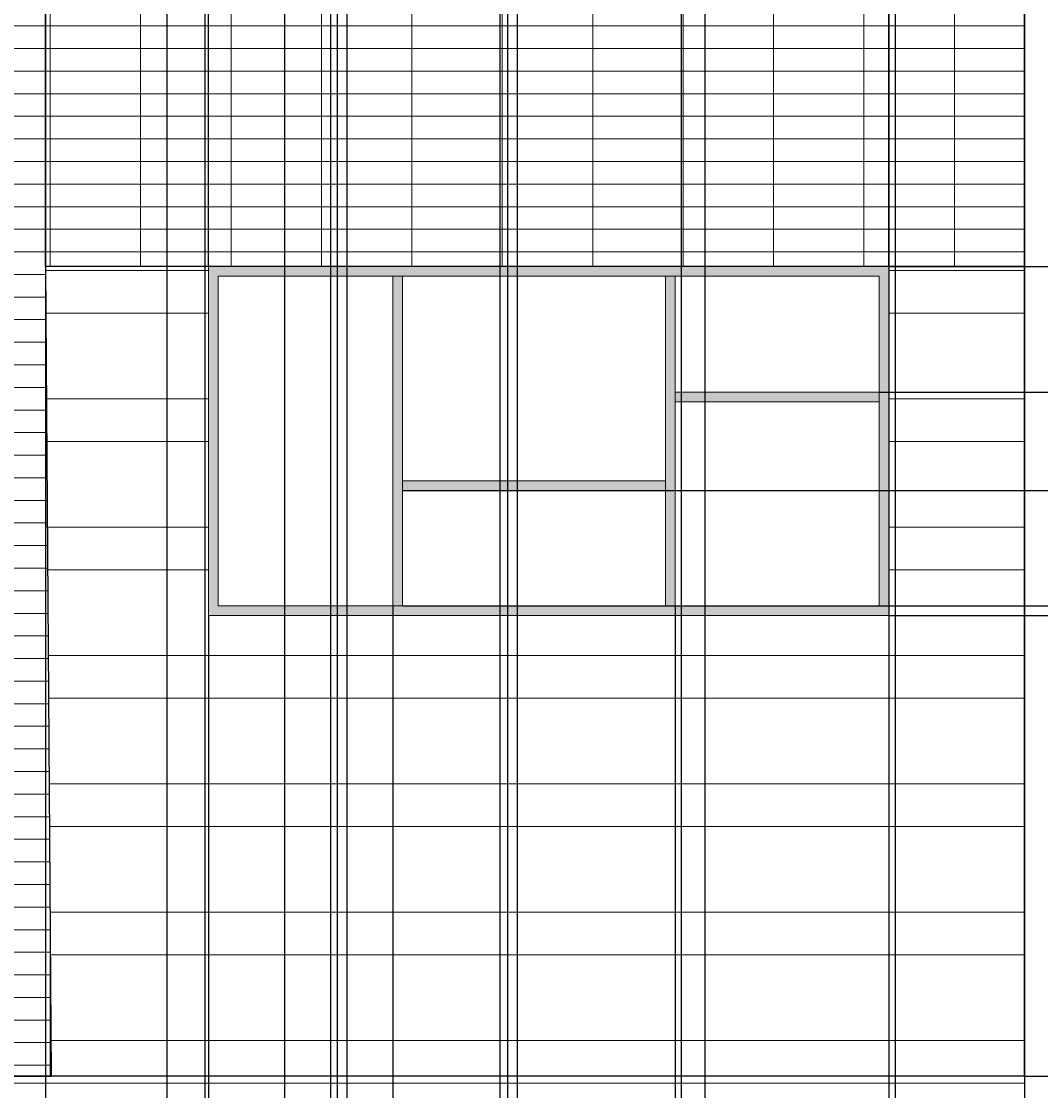
# Model space of a CAD drawing. Units: inches. Extents: x 241 to 943, y 109 to 1396.
# Tile 13 of 34: x 613 to 824, y 398 to 620. Entities that reach past the tile are written whole.
import ezdxf

# ---------------------------------------------------------------- set-up
doc = ezdxf.new("R2010")
doc.units = ezdxf.units.IN
doc.header["$MEASUREMENT"] = 0
for name, color, linetype, lineweight in [('A-ANNO-DIMS', 2, 'Continuous', 18), ('A-ELEV', 7, 'Continuous', 25), ('A-ELEV-SHAD', 9, 'Continuous', 13), ('A-GLAZ', 4, 'Continuous', 18), ('A-GLAZ-PATT', 18, 'Continuous', 13), ('A-WALL-PATT', 8, 'Continuous', 13)]:
    doc.layers.add(name, color=color, linetype=linetype, lineweight=lineweight)
doc.styles.get("Standard").update_dxf_attribs({"font": 'arial.ttf'})
doc.dimstyles.get("Standard").update_dxf_attribs({"dimtxt": 1.4375, "dimasz": 0.18, "dimexe": 0.18, "dimexo": 0.0625, "dimgap": 0.09, "dimtad": 0, "dimtih": 1, "dimtoh": 1, "dimdec": 4, "dimzin": 0, "dimdsep": 46, "dimlunit": 4, "dimtxsty": 'Standard', "dimcen": 0.09, "dimadec": 0, "dimazin": 0, "dimtfac": 1, "dimtdec": 4, "dimtofl": 0, "dimtmove": 0, "dimatfit": 3, "dimfxl": 1, "dimtolj": 1, "dimtzin": 0, "dimarcsym": 0})

# ---------------------------------------------------------------- blocks, each defined once
blk = doc.blocks.new('*D6')
at = {"layer": 'A-ANNO-DIMS', "color": 0, "lineweight": -2, "transparency": 16777216}
for p, q in [((820.84, 232.89), (820.84, 1395.05)), ((821.02, 1394.87), (848.73, 1394.87)), ((881.49, 1394.87), (853.77, 1394.87)), ((881.67, 232.89), (881.67, 1395.05))]:
    blk.add_line(p, q, dxfattribs=at)
at = {"layer": 'A-ANNO-DIMS', "color": 0, "transparency": 16777216}
for points in [[(821.02, 1394.9), (821.02, 1394.84), (820.84, 1394.87)], [(881.49, 1394.9), (881.49, 1394.84), (881.67, 1394.87)]]:
    blk.add_solid(points, dxfattribs=at)
at = {"layer": 'Defpoints', "color": 0, "transparency": 16777216}
for p in [(881.67, 1394.87), (820.84, 232.83), (881.67, 232.83)]:
    blk.add_point(p, dxfattribs=at)
at = {"layer": 'A-ANNO-DIMS', "color": 0, "transparency": 16777216, "insert": (851.25, 1394.87), "char_height": 1.438, "attachment_point": 5}
blk.add_mtext('\\A1;60.83', dxfattribs=at)
blk = doc.blocks.new('*D12')
at = {"layer": 'A-ANNO-DIMS', "color": 0, "lineweight": -2, "transparency": 16777216}
for p, q in [((530.23, 384.24), (530.23, 1395.05)), ((530.41, 1394.87), (587.56, 1394.87)), ((650.73, 1394.87), (593.58, 1394.87)), ((650.91, 384.24), (650.91, 1395.05))]:
    blk.add_line(p, q, dxfattribs=at)
at = {"layer": 'A-ANNO-DIMS', "color": 0, "transparency": 16777216}
for points in [[(530.41, 1394.9), (530.41, 1394.84), (530.23, 1394.87)], [(650.73, 1394.9), (650.73, 1394.84), (650.91, 1394.87)]]:
    blk.add_solid(points, dxfattribs=at)
at = {"layer": 'Defpoints', "color": 0, "transparency": 16777216}
for p in [(650.91, 1394.87), (530.23, 384.18), (650.91, 384.18)]:
    blk.add_point(p, dxfattribs=at)
at = {"layer": 'A-ANNO-DIMS', "color": 0, "transparency": 16777216, "insert": (590.57, 1394.87), "char_height": 1.438, "attachment_point": 5}
blk.add_mtext('\\A1;120.68', dxfattribs=at)
blk = doc.blocks.new('*D13')
at = {"layer": 'A-ANNO-DIMS', "color": 0, "lineweight": -2, "transparency": 16777216}
for p, q in [((650.91, 384.24), (650.91, 1395.05)), ((651.09, 1394.87), (656.14, 1394.87)), ((667.21, 1394.87), (662.16, 1394.87)), ((667.39, 290.06), (667.39, 1395.05))]:
    blk.add_line(p, q, dxfattribs=at)
at = {"layer": 'A-ANNO-DIMS', "color": 0, "transparency": 16777216}
for points in [[(651.09, 1394.9), (651.09, 1394.84), (650.91, 1394.87)], [(667.21, 1394.9), (667.21, 1394.84), (667.39, 1394.87)]]:
    blk.add_solid(points, dxfattribs=at)
at = {"layer": 'Defpoints', "color": 0, "transparency": 16777216}
for p in [(667.39, 1394.87), (650.91, 384.18), (667.39, 290)]:
    blk.add_point(p, dxfattribs=at)
at = {"layer": 'A-ANNO-DIMS', "color": 0, "transparency": 16777216, "insert": (659.15, 1394.87), "char_height": 1.438, "attachment_point": 5}
blk.add_mtext('\\A1;16.486', dxfattribs=at)
blk = doc.blocks.new('*D14')
at = {"layer": 'A-ANNO-DIMS', "color": 0, "lineweight": -2, "transparency": 16777216}
for p, q in [((667.39, 290.06), (667.39, 1395.05)), ((667.57, 1394.87), (727.7, 1394.87)), ((793.85, 1394.87), (733.72, 1394.87)), ((794.03, 290.06), (794.03, 1395.05))]:
    blk.add_line(p, q, dxfattribs=at)
at = {"layer": 'A-ANNO-DIMS', "color": 0, "transparency": 16777216}
for points in [[(667.57, 1394.9), (667.57, 1394.84), (667.39, 1394.87)], [(793.85, 1394.9), (793.85, 1394.84), (794.03, 1394.87)]]:
    blk.add_solid(points, dxfattribs=at)
at = {"layer": 'Defpoints', "color": 0, "transparency": 16777216}
for p in [(794.03, 1394.87), (667.39, 290), (794.03, 290)]:
    blk.add_point(p, dxfattribs=at)
at = {"layer": 'A-ANNO-DIMS', "color": 0, "transparency": 16777216, "insert": (730.71, 1394.87), "char_height": 1.438, "attachment_point": 5}
blk.add_mtext('\\A1;126.63', dxfattribs=at)
blk = doc.blocks.new('*D15')
at = {"layer": 'A-ANNO-DIMS', "color": 0, "lineweight": -2, "transparency": 16777216}
for p, q in [((794.03, 290.06), (794.03, 1395.05)), ((794.21, 1394.87), (805.04, 1394.87)), ((820.66, 1394.87), (809.82, 1394.87)), ((820.84, 232.89), (820.84, 1395.05))]:
    blk.add_line(p, q, dxfattribs=at)
at = {"layer": 'A-ANNO-DIMS', "color": 0, "transparency": 16777216}
for points in [[(794.21, 1394.9), (794.21, 1394.84), (794.03, 1394.87)], [(820.66, 1394.9), (820.66, 1394.84), (820.84, 1394.87)]]:
    blk.add_solid(points, dxfattribs=at)
at = {"layer": 'Defpoints', "color": 0, "transparency": 16777216}
for p in [(820.84, 1394.87), (794.03, 290), (820.84, 232.83)]:
    blk.add_point(p, dxfattribs=at)
at = {"layer": 'A-ANNO-DIMS', "color": 0, "transparency": 16777216, "insert": (807.43, 1394.87), "char_height": 1.438, "attachment_point": 5}
blk.add_mtext('\\A1;26.81', dxfattribs=at)
blk = doc.blocks.new('*D31')
at = {"layer": 'A-ANNO-DIMS', "color": 0, "lineweight": -2, "transparency": 16777216}
for p, q in [((792.75, 496.44), (940.6, 496.44)), ((940.42, 496.26), (940.42, 449.46)), ((940.42, 401.01), (940.42, 447.81)), ((820.9, 400.83), (940.6, 400.83))]:
    blk.add_line(p, q, dxfattribs=at)
at = {"layer": 'A-ANNO-DIMS', "color": 0, "transparency": 16777216}
for points in [[(940.39, 496.26), (940.45, 496.26), (940.42, 496.44)], [(940.39, 401.01), (940.45, 401.01), (940.42, 400.83)]]:
    blk.add_solid(points, dxfattribs=at)
at = {"layer": 'Defpoints', "color": 0, "transparency": 16777216}
for p in [(792.69, 496.44), (940.42, 496.44), (820.84, 400.83)]:
    blk.add_point(p, dxfattribs=at)
at = {"layer": 'A-ANNO-DIMS', "color": 0, "transparency": 16777216, "insert": (940.42, 448.63), "char_height": 1.438, "attachment_point": 5}
blk.add_mtext('\\A1;95.61', dxfattribs=at)
blk = doc.blocks.new('*D41')
at = {"layer": 'A-ANNO-DIMS', "color": 0, "lineweight": -2, "transparency": 16777216}
for p, q in [((820.77, 400.83), (244.31, 400.83)), ((244.49, 400.65), (244.49, 317.65)), ((244.49, 233.01), (244.49, 316.01)), ((820.77, 232.83), (244.31, 232.83))]:
    blk.add_line(p, q, dxfattribs=at)
at = {"layer": 'A-ANNO-DIMS', "color": 0, "transparency": 16777216}
for points in [[(244.46, 400.65), (244.52, 400.65), (244.49, 400.83)], [(244.46, 233.01), (244.52, 233.01), (244.49, 232.83)]]:
    blk.add_solid(points, dxfattribs=at)
at = {"layer": 'Defpoints', "color": 0, "transparency": 16777216}
for p in [(244.49, 400.83), (820.84, 400.83), (820.84, 232.83)]:
    blk.add_point(p, dxfattribs=at)
at = {"layer": 'A-ANNO-DIMS', "color": 0, "transparency": 16777216, "insert": (244.49, 316.83), "char_height": 1.438, "attachment_point": 5}
blk.add_mtext('\\A1;168', dxfattribs=at)
blk = doc.blocks.new('*D45')
at = {"layer": 'A-ANNO-DIMS', "color": 0, "lineweight": -2, "transparency": 16777216}
for p, q in [((792.75, 568.83), (940.6, 568.83)), ((940.42, 568.65), (940.42, 533.46)), ((940.42, 496.62), (940.42, 531.81)), ((792.75, 496.44), (940.6, 496.44))]:
    blk.add_line(p, q, dxfattribs=at)
at = {"layer": 'A-ANNO-DIMS', "color": 0, "transparency": 16777216}
for points in [[(940.39, 568.65), (940.45, 568.65), (940.42, 568.83)], [(940.39, 496.62), (940.45, 496.62), (940.42, 496.44)]]:
    blk.add_solid(points, dxfattribs=at)
at = {"layer": 'Defpoints', "color": 0, "transparency": 16777216}
for p in [(792.69, 568.83), (940.42, 568.83), (792.69, 496.44)]:
    blk.add_point(p, dxfattribs=at)
at = {"layer": 'A-ANNO-DIMS', "color": 0, "transparency": 16777216, "insert": (940.42, 532.63), "char_height": 1.438, "attachment_point": 5}
blk.add_mtext('\\A1;72.39', dxfattribs=at)
blk = doc.blocks.new('*D63')
at = {"layer": 'A-ANNO-DIMS', "color": 0, "lineweight": -2, "transparency": 16777216}
for p, q in [((651.6, 568.89), (651.6, 1395.05)), ((651.78, 1394.87), (719.84, 1394.87)), ((792.51, 1394.87), (724.45, 1394.87)), ((792.69, 568.89), (792.69, 1395.05))]:
    blk.add_line(p, q, dxfattribs=at)
at = {"layer": 'A-ANNO-DIMS', "color": 0, "transparency": 16777216}
for points in [[(651.78, 1394.9), (651.78, 1394.84), (651.6, 1394.87)], [(792.51, 1394.9), (792.51, 1394.84), (792.69, 1394.87)]]:
    blk.add_solid(points, dxfattribs=at)
at = {"layer": 'Defpoints', "color": 0, "transparency": 16777216}
for p in [(792.69, 1394.87), (651.6, 568.83), (792.69, 568.83)]:
    blk.add_point(p, dxfattribs=at)
at = {"layer": 'A-ANNO-DIMS', "color": 0, "transparency": 16777216, "insert": (722.14, 1394.87), "char_height": 1.438, "attachment_point": 5}
blk.add_mtext('\\A1;141.1', dxfattribs=at)
blk = doc.blocks.new('*D64')
at = {"layer": 'A-ANNO-DIMS', "color": 0, "lineweight": -2, "transparency": 16777216}
for p, q in [((792.69, 568.89), (792.69, 1395.05)), ((792.87, 1394.87), (803.68, 1394.87)), ((820.66, 1394.87), (809.85, 1394.87)), ((820.84, 568.89), (820.84, 1395.05))]:
    blk.add_line(p, q, dxfattribs=at)
at = {"layer": 'A-ANNO-DIMS', "color": 0, "transparency": 16777216}
for points in [[(792.87, 1394.9), (792.87, 1394.84), (792.69, 1394.87)], [(820.66, 1394.9), (820.66, 1394.84), (820.84, 1394.87)]]:
    blk.add_solid(points, dxfattribs=at)
at = {"layer": 'Defpoints', "color": 0, "transparency": 16777216}
for p in [(820.84, 1394.87), (792.69, 568.83), (820.84, 568.83)]:
    blk.add_point(p, dxfattribs=at)
at = {"layer": 'A-ANNO-DIMS', "color": 0, "transparency": 16777216, "insert": (806.76, 1394.87), "char_height": 1.438, "attachment_point": 5}
blk.add_mtext('\\A1;28.146', dxfattribs=at)
blk = doc.blocks.new('*D82')
at = {"layer": 'A-ANNO-DIMS', "color": 0, "lineweight": -2, "transparency": 16777216}
for p, q in [((565.2, 568.89), (565.2, 1395.05)), ((565.38, 1394.87), (605.89, 1394.87)), ((651.42, 1394.87), (610.91, 1394.87)), ((651.6, 568.89), (651.6, 1395.05))]:
    blk.add_line(p, q, dxfattribs=at)
at = {"layer": 'A-ANNO-DIMS', "color": 0, "transparency": 16777216}
for points in [[(565.38, 1394.9), (565.38, 1394.84), (565.2, 1394.87)], [(651.42, 1394.9), (651.42, 1394.84), (651.6, 1394.87)]]:
    blk.add_solid(points, dxfattribs=at)
at = {"layer": 'Defpoints', "color": 0, "transparency": 16777216}
for p in [(651.6, 1394.87), (565.2, 568.83), (651.6, 568.83)]:
    blk.add_point(p, dxfattribs=at)
at = {"layer": 'A-ANNO-DIMS', "color": 0, "transparency": 16777216, "insert": (608.4, 1394.87), "char_height": 1.438, "attachment_point": 5}
blk.add_mtext('\\A1;86.40', dxfattribs=at)
blk = doc.blocks.new('*D85')
at = {"layer": 'A-ANNO-DIMS', "color": 0, "lineweight": -2, "transparency": 16777216}
for p, q in [((749.7, 626.4), (940.6, 626.4)), ((940.42, 626.22), (940.42, 598.44)), ((940.42, 569.01), (940.42, 596.79)), ((792.75, 568.83), (940.6, 568.83))]:
    blk.add_line(p, q, dxfattribs=at)
at = {"layer": 'A-ANNO-DIMS', "color": 0, "transparency": 16777216}
for points in [[(940.39, 626.22), (940.45, 626.22), (940.42, 626.4)], [(940.39, 569.01), (940.45, 569.01), (940.42, 568.83)]]:
    blk.add_solid(points, dxfattribs=at)
at = {"layer": 'Defpoints', "color": 0, "transparency": 16777216}
for p in [(749.63, 626.4), (940.42, 626.4), (792.69, 568.83)]:
    blk.add_point(p, dxfattribs=at)
at = {"layer": 'A-ANNO-DIMS', "color": 0, "transparency": 16777216, "insert": (940.42, 597.62), "char_height": 1.438, "attachment_point": 5}
blk.add_mtext('\\A1;57.57', dxfattribs=at)
blk = doc.blocks.new('*D99')
at = {"layer": 'A-ANNO-DIMS', "color": 0, "lineweight": -2, "transparency": 16777216}
for p, q in [((417.09, 181.71), (417.09, 1395.05)), ((417.27, 1394.87), (539.16, 1394.87)), ((667.21, 1394.87), (545.33, 1394.87)), ((667.39, 214.58), (667.39, 1395.05))]:
    blk.add_line(p, q, dxfattribs=at)
at = {"layer": 'A-ANNO-DIMS', "color": 0, "transparency": 16777216}
for points in [[(417.27, 1394.9), (417.27, 1394.84), (417.09, 1394.87)], [(667.21, 1394.9), (667.21, 1394.84), (667.39, 1394.87)]]:
    blk.add_solid(points, dxfattribs=at)
at = {"layer": 'Defpoints', "color": 0, "transparency": 16777216}
for p in [(667.39, 1394.87), (667.39, 214.52), (417.09, 181.65)]:
    blk.add_point(p, dxfattribs=at)
at = {"layer": 'A-ANNO-DIMS', "color": 0, "transparency": 16777216, "insert": (542.24, 1394.87), "char_height": 1.438, "attachment_point": 5}
blk.add_mtext('\\A1;250.30', dxfattribs=at)
blk = doc.blocks.new('*D119')
at = {"layer": 'A-ANNO-DIMS', "color": 0, "lineweight": -2, "transparency": 16777216}
for p, q in [((617.76, 734.79), (617.76, 109.81)), ((642.92, 734.79), (642.92, 109.81)), ((617.94, 109.99), (627.81, 109.99)), ((642.74, 109.99), (632.87, 109.99))]:
    blk.add_line(p, q, dxfattribs=at)
at = {"layer": 'A-ANNO-DIMS', "color": 0, "transparency": 16777216}
for points in [[(617.94, 110.02), (617.94, 109.96), (617.76, 109.99)], [(642.74, 110.02), (642.74, 109.96), (642.92, 109.99)]]:
    blk.add_solid(points, dxfattribs=at)
at = {"layer": 'Defpoints', "color": 0, "transparency": 16777216}
for p in [(617.76, 734.85), (642.92, 734.85), (642.92, 109.99)]:
    blk.add_point(p, dxfattribs=at)
at = {"layer": 'A-ANNO-DIMS', "color": 0, "transparency": 16777216, "insert": (630.34, 109.99), "char_height": 1.438, "attachment_point": 5}
blk.add_mtext('\\A1;25.16', dxfattribs=at)
blk = doc.blocks.new('*D120')
at = {"layer": 'A-ANNO-DIMS', "color": 0, "lineweight": -2, "transparency": 16777216}
for p, q in [((642.92, 734.79), (642.92, 109.81)), ((678.27, 734.79), (678.27, 109.81)), ((643.1, 109.99), (658.07, 109.99)), ((678.09, 109.99), (663.11, 109.99))]:
    blk.add_line(p, q, dxfattribs=at)
at = {"layer": 'A-ANNO-DIMS', "color": 0, "transparency": 16777216}
for points in [[(643.1, 110.02), (643.1, 109.96), (642.92, 109.99)], [(678.09, 110.02), (678.09, 109.96), (678.27, 109.99)]]:
    blk.add_solid(points, dxfattribs=at)
at = {"layer": 'Defpoints', "color": 0, "transparency": 16777216}
for p in [(642.92, 734.85), (678.27, 734.85), (678.27, 109.99)]:
    blk.add_point(p, dxfattribs=at)
at = {"layer": 'A-ANNO-DIMS', "color": 0, "transparency": 16777216, "insert": (660.59, 109.99), "char_height": 1.438, "attachment_point": 5}
blk.add_mtext('\\A1;35.35', dxfattribs=at)
blk = doc.blocks.new('*D121')
at = {"layer": 'A-ANNO-DIMS', "color": 0, "lineweight": -2, "transparency": 16777216}
for p, q in [((680.27, 736.86), (680.27, 109.81)), ((713.62, 736.86), (713.62, 109.81)), ((680.45, 109.99), (693.87, 109.99)), ((713.44, 109.99), (700.02, 109.99))]:
    blk.add_line(p, q, dxfattribs=at)
at = {"layer": 'A-ANNO-DIMS', "color": 0, "transparency": 16777216}
for points in [[(680.45, 110.02), (680.45, 109.96), (680.27, 109.99)], [(713.44, 110.02), (713.44, 109.96), (713.62, 109.99)]]:
    blk.add_solid(points, dxfattribs=at)
at = {"layer": 'Defpoints', "color": 0, "transparency": 16777216}
for p in [(680.27, 736.92), (713.62, 736.92), (713.62, 109.99)]:
    blk.add_point(p, dxfattribs=at)
at = {"layer": 'A-ANNO-DIMS', "color": 0, "transparency": 16777216, "insert": (696.95, 109.99), "char_height": 1.438, "attachment_point": 5}
blk.add_mtext('\\A1;33.356', dxfattribs=at)
blk = doc.blocks.new('*D122')
at = {"layer": 'A-ANNO-DIMS', "color": 0, "lineweight": -2, "transparency": 16777216}
for p, q in [((715.62, 734.79), (715.62, 109.81)), ((754.54, 734.79), (754.54, 109.81)), ((715.8, 109.99), (732.7, 109.99)), ((754.36, 109.99), (737.46, 109.99))]:
    blk.add_line(p, q, dxfattribs=at)
at = {"layer": 'A-ANNO-DIMS', "color": 0, "transparency": 16777216}
for points in [[(715.8, 110.02), (715.8, 109.96), (715.62, 109.99)], [(754.36, 110.02), (754.36, 109.96), (754.54, 109.99)]]:
    blk.add_solid(points, dxfattribs=at)
at = {"layer": 'Defpoints', "color": 0, "transparency": 16777216}
for p in [(715.62, 734.85), (754.54, 734.85), (754.54, 109.99)]:
    blk.add_point(p, dxfattribs=at)
at = {"layer": 'A-ANNO-DIMS', "color": 0, "transparency": 16777216, "insert": (735.08, 109.99), "char_height": 1.438, "attachment_point": 5}
blk.add_mtext('\\A1;38.91', dxfattribs=at)
blk = doc.blocks.new('*D123')
at = {"layer": 'A-ANNO-DIMS', "color": 0, "lineweight": -2, "transparency": 16777216}
for p, q in [((754.54, 734.79), (754.54, 109.81)), ((792.69, 734.79), (792.69, 109.81)), ((754.72, 109.99), (771.09, 109.99)), ((792.51, 109.99), (776.13, 109.99))]:
    blk.add_line(p, q, dxfattribs=at)
at = {"layer": 'A-ANNO-DIMS', "color": 0, "transparency": 16777216}
for points in [[(754.72, 110.02), (754.72, 109.96), (754.54, 109.99)], [(792.51, 110.02), (792.51, 109.96), (792.69, 109.99)]]:
    blk.add_solid(points, dxfattribs=at)
at = {"layer": 'Defpoints', "color": 0, "transparency": 16777216}
for p in [(754.54, 734.85), (792.69, 734.85), (792.69, 109.99)]:
    blk.add_point(p, dxfattribs=at)
at = {"layer": 'A-ANNO-DIMS', "color": 0, "transparency": 16777216, "insert": (773.61, 109.99), "char_height": 1.438, "attachment_point": 5}
blk.add_mtext('\\A1;38.15', dxfattribs=at)
blk = doc.blocks.new('*D132')
at = {"layer": 'A-ANNO-DIMS', "color": 0, "lineweight": -2, "transparency": 16777216}
for p, q in [((676.87, 628.34), (676.87, 109.81)), ((617.76, 626.34), (617.76, 109.81)), ((617.94, 109.99), (644.94, 109.99)), ((676.69, 109.99), (649.69, 109.99))]:
    blk.add_line(p, q, dxfattribs=at)
at = {"layer": 'A-ANNO-DIMS', "color": 0, "transparency": 16777216}
for points in [[(617.94, 110.02), (617.94, 109.96), (617.76, 109.99)], [(676.69, 110.02), (676.69, 109.96), (676.87, 109.99)]]:
    blk.add_solid(points, dxfattribs=at)
at = {"layer": 'Defpoints', "color": 0, "transparency": 16777216}
for p in [(676.87, 628.4), (617.76, 626.4), (676.87, 109.99)]:
    blk.add_point(p, dxfattribs=at)
at = {"layer": 'A-ANNO-DIMS', "color": 0, "transparency": 16777216, "insert": (647.31, 109.99), "char_height": 1.438, "attachment_point": 5}
blk.add_mtext('\\A1;59.11', dxfattribs=at)
blk = doc.blocks.new('*D133')
at = {"layer": 'A-ANNO-DIMS', "color": 0, "lineweight": -2, "transparency": 16777216}
for p, q in [((676.87, 628.34), (676.87, 109.81)), ((712.02, 628.34), (712.02, 109.81)), ((677.05, 109.99), (691.92, 109.99)), ((711.84, 109.99), (696.96, 109.99))]:
    blk.add_line(p, q, dxfattribs=at)
at = {"layer": 'A-ANNO-DIMS', "color": 0, "transparency": 16777216}
for points in [[(677.05, 110.02), (677.05, 109.96), (676.87, 109.99)], [(711.84, 110.02), (711.84, 109.96), (712.02, 109.99)]]:
    blk.add_solid(points, dxfattribs=at)
at = {"layer": 'Defpoints', "color": 0, "transparency": 16777216}
for p in [(676.87, 628.4), (712.02, 628.4), (712.02, 109.99)]:
    blk.add_point(p, dxfattribs=at)
at = {"layer": 'A-ANNO-DIMS', "color": 0, "transparency": 16777216, "insert": (694.44, 109.99), "char_height": 1.438, "attachment_point": 5}
blk.add_mtext('\\A1;35.15', dxfattribs=at)
blk = doc.blocks.new('*D134')
at = {"layer": 'A-ANNO-DIMS', "color": 0, "lineweight": -2, "transparency": 16777216}
for p, q in [((712.02, 628.34), (712.02, 109.81)), ((749.63, 626.34), (749.63, 109.81)), ((712.2, 109.99), (727.75, 109.99)), ((749.45, 109.99), (733.9, 109.99))]:
    blk.add_line(p, q, dxfattribs=at)
at = {"layer": 'A-ANNO-DIMS', "color": 0, "transparency": 16777216}
for points in [[(712.2, 110.02), (712.2, 109.96), (712.02, 109.99)], [(749.45, 110.02), (749.45, 109.96), (749.63, 109.99)]]:
    blk.add_solid(points, dxfattribs=at)
at = {"layer": 'Defpoints', "color": 0, "transparency": 16777216}
for p in [(712.02, 628.4), (749.63, 626.4), (749.63, 109.99)]:
    blk.add_point(p, dxfattribs=at)
at = {"layer": 'A-ANNO-DIMS', "color": 0, "transparency": 16777216, "insert": (730.82, 109.99), "char_height": 1.438, "attachment_point": 5}
blk.add_mtext('\\A1;37.616', dxfattribs=at)
blk = doc.blocks.new('*D142')
at = {"layer": 'A-ANNO-DIMS', "color": 0, "lineweight": -2, "transparency": 16777216}
for p, q in [((689.79, 498.38), (689.79, 109.81)), ((651.6, 496.38), (651.6, 109.81)), ((651.78, 109.99), (668.18, 109.99)), ((689.61, 109.99), (673.21, 109.99))]:
    blk.add_line(p, q, dxfattribs=at)
at = {"layer": 'A-ANNO-DIMS', "color": 0, "transparency": 16777216}
for points in [[(651.78, 110.02), (651.78, 109.96), (651.6, 109.99)], [(689.61, 110.02), (689.61, 109.96), (689.79, 109.99)]]:
    blk.add_solid(points, dxfattribs=at)
at = {"layer": 'Defpoints', "color": 0, "transparency": 16777216}
for p in [(689.79, 498.44), (651.6, 496.44), (689.79, 109.99)]:
    blk.add_point(p, dxfattribs=at)
at = {"layer": 'A-ANNO-DIMS', "color": 0, "transparency": 16777216, "insert": (670.7, 109.99), "char_height": 1.438, "attachment_point": 5}
blk.add_mtext('\\A1;38.20', dxfattribs=at)
blk = doc.blocks.new('*D143')
at = {"layer": 'A-ANNO-DIMS', "color": 0, "lineweight": -2, "transparency": 16777216}
for p, q in [((689.79, 498.38), (689.79, 109.81)), ((748.33, 498.38), (748.33, 109.81)), ((689.97, 109.99), (716.55, 109.99)), ((748.15, 109.99), (721.58, 109.99))]:
    blk.add_line(p, q, dxfattribs=at)
at = {"layer": 'A-ANNO-DIMS', "color": 0, "transparency": 16777216}
for points in [[(689.97, 110.02), (689.97, 109.96), (689.79, 109.99)], [(748.15, 110.02), (748.15, 109.96), (748.33, 109.99)]]:
    blk.add_solid(points, dxfattribs=at)
at = {"layer": 'Defpoints', "color": 0, "transparency": 16777216}
for p in [(689.79, 498.44), (748.33, 498.44), (748.33, 109.99)]:
    blk.add_point(p, dxfattribs=at)
at = {"layer": 'A-ANNO-DIMS', "color": 0, "transparency": 16777216, "insert": (719.06, 109.99), "char_height": 1.438, "attachment_point": 5}
blk.add_mtext('\\A1;58.54', dxfattribs=at)
blk = doc.blocks.new('*D144')
at = {"layer": 'A-ANNO-DIMS', "color": 0, "lineweight": -2, "transparency": 16777216}
for p, q in [((748.33, 498.38), (748.33, 109.81)), ((792.69, 496.38), (792.69, 109.81)), ((748.51, 109.99), (767.97, 109.99)), ((792.51, 109.99), (773.06, 109.99))]:
    blk.add_line(p, q, dxfattribs=at)
at = {"layer": 'A-ANNO-DIMS', "color": 0, "transparency": 16777216}
for points in [[(748.51, 110.02), (748.51, 109.96), (748.33, 109.99)], [(792.51, 110.02), (792.51, 109.96), (792.69, 109.99)]]:
    blk.add_solid(points, dxfattribs=at)
at = {"layer": 'Defpoints', "color": 0, "transparency": 16777216}
for p in [(748.33, 498.44), (792.69, 496.44), (792.69, 109.99)]:
    blk.add_point(p, dxfattribs=at)
at = {"layer": 'A-ANNO-DIMS', "color": 0, "transparency": 16777216, "insert": (770.51, 109.99), "char_height": 1.438, "attachment_point": 5}
blk.add_mtext('\\A1;44.36', dxfattribs=at)
blk = doc.blocks.new('*D145')
at = {"layer": 'A-ANNO-DIMS', "color": 0, "lineweight": -2, "transparency": 16777216}
for p, q in [((691.86, 522.37), (940.6, 522.37)), ((940.42, 522.19), (940.42, 511.23)), ((940.42, 498.62), (940.42, 509.58)), ((691.86, 498.44), (940.6, 498.44))]:
    blk.add_line(p, q, dxfattribs=at)
at = {"layer": 'A-ANNO-DIMS', "color": 0, "transparency": 16777216}
for points in [[(940.39, 522.19), (940.45, 522.19), (940.42, 522.37)], [(940.39, 498.62), (940.45, 498.62), (940.42, 498.44)]]:
    blk.add_solid(points, dxfattribs=at)
at = {"layer": 'Defpoints', "color": 0, "transparency": 16777216}
for p in [(691.79, 522.37), (940.42, 522.37), (691.79, 498.44)]:
    blk.add_point(p, dxfattribs=at)
at = {"layer": 'A-ANNO-DIMS', "color": 0, "transparency": 16777216, "insert": (940.42, 510.41), "char_height": 1.438, "attachment_point": 5}
blk.add_mtext('\\A1;23.933', dxfattribs=at)
blk = doc.blocks.new('*D146')
at = {"layer": 'A-ANNO-DIMS', "color": 0, "lineweight": -2, "transparency": 16777216}
for p, q in [((790.75, 542.8), (940.6, 542.8)), ((940.42, 542.62), (940.42, 521.44)), ((940.42, 498.62), (940.42, 519.8)), ((790.75, 498.44), (940.6, 498.44))]:
    blk.add_line(p, q, dxfattribs=at)
at = {"layer": 'A-ANNO-DIMS', "color": 0, "transparency": 16777216}
for points in [[(940.39, 542.62), (940.45, 542.62), (940.42, 542.8)], [(940.39, 498.62), (940.45, 498.62), (940.42, 498.44)]]:
    blk.add_solid(points, dxfattribs=at)
at = {"layer": 'Defpoints', "color": 0, "transparency": 16777216}
for p in [(790.69, 542.8), (940.42, 542.8), (790.69, 498.44)]:
    blk.add_point(p, dxfattribs=at)
at = {"layer": 'A-ANNO-DIMS', "color": 0, "transparency": 16777216, "insert": (940.42, 520.62), "char_height": 1.438, "attachment_point": 5}
blk.add_mtext('\\A1;44.36', dxfattribs=at)

msp = doc.modelspace()

# ---------------------------------------------------------------- hatches: boundary and pattern name
at = {"layer": 'A-ELEV-SHAD'}
h = msp.add_hatch(color=256, dxfattribs=at)
h.dxf.hatch_style = 1
h.paths.add_polyline_path([(748.3325, 566.8295), (746.3325, 566.8295), (746.3325, 498.4395), (748.3325, 498.4395)])
h.paths.add_polyline_path([(746.3325, 524.3723), (691.794, 524.3723), (691.794, 522.3723), (746.3325, 522.3723)])
h.paths.add_polyline_path([(691.794, 566.8295), (689.794, 566.8295), (689.794, 498.4395), (691.794, 498.4395)])
h.paths.add_polyline_path([(790.691, 542.7994), (748.3325, 542.7994), (748.3325, 540.7994), (790.691, 540.7994)])
h.paths.add_polyline_path([(500.3323, 384.1784), (479.596, 384.1784), (479.596, 289.6933), (500.3323, 289.6933)])
h.paths.add_polyline_path([(481.596, 291.6933), (481.596, 382.1784), (498.3323, 382.1784), (498.3323, 291.6933)], flags=16)
h.paths.add_polyline_path([(462.1074, 384.1784), (390.895, 384.1784), (390.895, 289.6933), (462.1074, 289.6933)])
h.paths.add_polyline_path([(392.895, 291.6933), (392.895, 382.1784), (460.1074, 382.1784), (460.1074, 291.6933)], flags=16)
h.paths.add_polyline_path([(794.0275, 289.9984), (667.3935, 289.9984), (667.3935, 214.5189), (794.0275, 214.5189)])
h.paths.add_polyline_path([(792.0275, 287.9984), (792.0275, 216.5189), (669.3935, 216.5189), (669.3935, 287.9984)], flags=16)
h.paths.add_polyline_path([(508.0803, 525.3816), (506.0803, 525.3816), (506.0803, 521.3754), (452.9259, 521.3754), (452.9259, 525.3816), (450.9259, 525.3816), (450.9259, 519.3754), (508.0803, 519.3754)], flags=0)
h.paths.add_polyline_path([(508.0803, 566.8295), (450.9259, 566.8295), (450.9259, 527.3816), (452.9259, 527.3816), (452.9259, 564.8295), (506.0803, 564.8295), (506.0803, 527.3816), (508.0803, 527.3816)], flags=0)
h.paths.add_polyline_path([(537.4269, 566.8295), (534.1778, 566.8295), (534.1778, 527.3816), (537.4269, 527.3816)], flags=0)
h.paths.add_polyline_path([(537.4269, 525.3816), (534.1778, 525.3816), (534.1778, 508.9074), (537.4269, 508.9074)], flags=0)
h.paths.add_polyline_path([(565.2023, 568.8295), (424.1086, 568.8295), (424.1086, 496.4395), (565.2023, 496.4395)])
h.paths.add_polyline_path([(563.2023, 508.9074), (563.2023, 498.4395), (426.1086, 498.4395), (426.1086, 566.8295), (563.2023, 566.8295)], flags=16)
h.paths.add_polyline_path([(508.0803, 508.9074), (508.0803, 519.3754), (450.9259, 519.3754), (450.9259, 525.3816), (445.5808, 525.3816, -1), (445.5808, 527.3816), (450.9259, 527.3816), (450.9259, 566.8295), (508.0803, 566.8295), (537.4269, 566.8295), (537.4269, 508.9074)], flags=0)
h.paths.add_polyline_path([(506.0803, 521.3754), (452.9259, 521.3754), (452.9259, 564.8295), (506.0803, 564.8295)], flags=0)
h = msp.add_hatch(color=256, dxfattribs=at)
h.dxf.hatch_style = 1
h.paths.add_polyline_path([(691.794, 566.8295), (689.794, 566.8295), (689.794, 498.4395), (691.794, 498.4395)], flags=0)
h.paths.add_polyline_path([(792.691, 568.8295), (651.5974, 568.8295), (651.5974, 496.4395), (792.691, 496.4395)])
h.paths.add_polyline_path([(790.691, 566.8295), (790.691, 498.4395), (653.5974, 498.4395), (653.5974, 566.8295)], flags=16)
h.paths.add_polyline_path([(691.794, 524.3723), (746.3325, 524.3723), (746.3325, 522.3723), (691.794, 522.3723)], flags=0)
h.paths.add_polyline_path([(746.3325, 524.3723), (691.794, 524.3723), (691.794, 522.3723), (746.3325, 522.3723)], flags=0)
h.paths.add_polyline_path([(748.3325, 566.8295), (746.3325, 566.8295), (746.3325, 498.4395), (748.3325, 498.4395)], flags=0)
at = {"layer": 'A-GLAZ-PATT'}
h = msp.add_hatch(dxfattribs=at)
h.set_pattern_fill('ANSI31', color=256, scale=34, angle=45)
h.paths.add_polyline_path([(486.3418, 786.9154), (413.1187, 786.9154), (413.1187, 761.2284), (486.3418, 761.2284)])
h.paths.add_polyline_path([(486.3418, 954.9154), (413.1187, 954.9154), (413.1187, 929.2284), (486.3418, 929.2284)])
h.paths.add_polyline_path([(462.1074, 289.6933), (390.895, 289.6933), (390.895, 277.4626), (390.895, 274.3507), (462.1074, 274.3507), (462.1074, 277.4626)])
h.paths.add_polyline_path([(500.3323, 289.6933), (479.596, 289.6933), (479.596, 274.3507), (500.3323, 274.3507)])
h.paths.add_polyline_path([(450.9259, 566.8295), (426.1086, 566.8295), (426.1086, 498.4395), (446.4348, 498.4395), (446.4348, 519.3754), (450.9259, 519.3754), (450.9259, 525.3816), (445.5808, 525.3816, -1), (445.5808, 527.3816), (450.9259, 527.3816)])
h.paths.add_polyline_path([(563.2023, 508.9074), (534.1778, 508.9074), (508.1906, 508.9074), (508.1906, 498.4395), (563.2023, 498.4395)])
h.paths.add_polyline_path([(747.6328, 700.7912), (712.0171, 700.7912), (712.0171, 628.4013), (747.6328, 628.4013)])
h.paths.add_polyline_path([(446.4348, 643.7483), (426.1086, 643.7483), (426.1086, 630.4013), (446.4348, 630.4013)])
h.paths.add_polyline_path([(564.8076, 841.5382), (553.5166, 841.5382), (508.3064, 841.5382), (508.3064, 782.5808), (564.8076, 782.5808)])
h.paths.add_polyline_path([(564.8076, 780.5808), (508.3064, 780.5808), (508.3064, 773.4916), (564.8076, 773.4916)])
h.paths.add_polyline_path([(792.691, 762.5799), (759.6248, 762.5799), (759.6248, 736.9235), (759.6248, 734.8538), (792.691, 734.8538)])
h.paths.add_polyline_path([(564.8076, 1009.5382), (553.5166, 1009.5382), (508.3064, 1009.5382), (508.3064, 950.5808), (562.3033, 950.5808, -1), (562.3033, 948.5808), (508.3064, 948.5808), (508.3064, 941.4916), (564.8076, 941.4916)])
h.paths.add_polyline_path([(486.3418, 1122.9154), (413.1187, 1122.9154), (413.1187, 1097.2284), (486.3418, 1097.2284)])
at = {"layer": 'A-WALL-PATT'}
h = msp.add_hatch(dxfattribs=at)
h.set_pattern_fill('GRATE', color=256, scale=150)
h.paths.add_polyline_path([(747.7579, 1238.8538), (747.7579, 1275.9142), (747.7579, 1336.1154), (508.3064, 1336.1154), (508.3064, 1275.9142), (508.3064, 1238.8538), (508.3064, 1177.5382), (508.3064, 1109.4916), (508.3064, 1070.8538), (553.5166, 1070.8538), (749.6328, 1070.8538)])
h.paths.add_polyline_path([(533.952, 1108.1686), (533.952, 1177.7336), (533.952, 1303.0286), (724.819, 1303.0286), (724.819, 1108.1686)], flags=16)
h.paths.add_polyline_path([(535.952, 1110.1686), (535.952, 1175.7336), (722.819, 1175.7336), (722.819, 1110.1686)], flags=0)
h.paths.add_polyline_path([(643.4534, 1134.0739), (622.521, 1134.0739), (622.521, 1136.0739), (643.4534, 1136.0739)], flags=0)
h.paths.add_polyline_path([(617.7594, 568.8295), (617.7594, 734.8538), (377.0391, 734.8538), (377.0391, 566.8538), (377.0391, 400.8295), (417.0913, 400.8295), (618.9643, 400.8295)])
h.paths.add_polyline_path([(424.1086, 496.4395), (424.1086, 568.8295), (565.2023, 568.8295), (565.2023, 496.4395)], flags=16)
h.paths.add_polyline_path([(426.1086, 498.4395), (426.1086, 566.8295), (563.2023, 566.8295), (563.2023, 508.9074), (563.2023, 498.4395)], flags=0)
h.paths.add_polyline_path([(508.0803, 508.9074), (508.0803, 519.3754), (450.9259, 519.3754), (450.9259, 525.3816), (445.5808, 525.3816, -1), (445.5808, 527.3816), (450.9259, 527.3816), (450.9259, 566.8295), (508.0803, 566.8295), (537.4269, 566.8295), (537.4269, 508.9074)], flags=0)
h.paths.add_polyline_path([(506.0803, 521.3754), (452.9259, 521.3754), (452.9259, 564.8295), (506.0803, 564.8295)], flags=0)
h.paths.add_polyline_path([(424.1086, 628.4013), (424.1086, 700.7912), (592.9542, 700.7912), (592.9542, 628.4013)], flags=16)
h.paths.add_polyline_path([(426.1086, 630.4013), (426.1086, 698.7912), (590.8792, 698.7912), (590.8792, 630.4013)], flags=0)
h.paths.add_polyline_path([(508.1906, 651.3371), (508.0803, 651.3371), (450.9259, 651.3371), (428.0291, 651.3371), (428.0291, 698.7912), (451.9767, 698.7912), (508.0803, 698.7912), (537.4269, 698.7912), (563.2023, 698.7912), (563.2023, 659.3434), (563.9297, 659.3434), (563.9297, 651.3371)], flags=0)
h.paths.add_polyline_path([(506.0803, 653.3371), (452.9259, 653.3371), (452.9259, 657.3434), (445.5808, 657.3434, -1), (445.5808, 659.3434), (452.9259, 659.3434), (452.9259, 696.7912), (506.0803, 696.7912)], flags=0)
h = msp.add_hatch(dxfattribs=at)
h.set_pattern_fill('GRATE', color=256, scale=150)
h.paths.add_polyline_path([(820.8374, 1070.8538), (749.6328, 1070.8538), (553.5166, 1070.8538), (508.3064, 1070.8538), (508.3064, 1009.5382), (553.5166, 1009.5382), (564.8076, 1009.5382), (603.8694, 1009.5382), (751.5078, 1009.5382), (751.5078, 902.8538), (603.8694, 902.8538), (603.8694, 1009.5382), (564.8076, 1009.5382), (564.8076, 941.4916), (568.1348, 941.4916), (568.1348, 902.8538), (581.3632, 902.8538), (581.3632, 841.5382), (564.8076, 841.5382), (564.8076, 782.5808), (605.9087, 782.5808, -1), (605.9087, 780.5808), (564.8076, 780.5808), (564.8076, 773.4916), (597.514, 773.4916), (607.8162, 773.4916), (607.8162, 734.8538), (617.7594, 734.8538), (617.7594, 841.5382), (792.691, 841.5382), (792.691, 734.8538), (617.7594, 734.8538), (617.7594, 702.7912), (749.6328, 702.7912), (749.6328, 626.4013), (617.7594, 626.4013), (617.7594, 568.8295), (820.8374, 568.8295), (820.8374, 736.8295), (820.8374, 902.8538)])
h = msp.add_hatch(dxfattribs=at)
h.set_pattern_fill('ANSI32', color=256, scale=71, angle=135)
h.paths.add_polyline_path([(820.8374, 568.8295), (792.691, 568.8295), (792.691, 496.4395), (651.5974, 496.4395), (651.5974, 568.8295), (617.7594, 568.8295), (618.9643, 400.8295), (417.0913, 400.8295), (377.0391, 400.8295), (377.0391, 398.8538), (377.0391, 396.8782), (377.0391, 228.8782), (377.0391, 177.6977), (416.5078, 181.5724), (417.0913, 181.649), (530.2303, 196.5065), (530.2303, 384.1784), (650.907, 384.1784), (651.7861, 212.4693), (667.3935, 214.5189), (667.3935, 289.9984), (794.0275, 289.9984), (794.0275, 232.8295), (820.8374, 232.8295), (820.8374, 400.8295)])
h.paths.add_polyline_path([(500.3323, 384.1784), (500.3323, 289.6933), (500.3323, 274.3507), (479.596, 274.3507), (479.596, 289.6933), (479.596, 384.1784)], flags=16)
h.paths.add_polyline_path([(498.3323, 382.1784), (498.3323, 291.6933), (481.596, 291.6933), (481.596, 382.1784)], flags=0)
h.paths.add_polyline_path([(462.1074, 384.1784), (462.1074, 289.6933), (462.1074, 277.4626), (462.1074, 274.3507), (390.895, 274.3507), (390.895, 277.4626), (390.895, 289.6933), (390.895, 384.1784)], flags=16)
h.paths.add_polyline_path([(460.1074, 382.1784), (460.1074, 291.6933), (392.895, 291.6933), (392.895, 382.1784)], flags=0)
h.paths.add_polyline_path([(595.3136, 372.9401), (641.6196, 372.9401), (641.6196, 246.4081), (651.6121, 246.4593), (650.907, 384.1784), (530.2303, 384.1784), (530.2303, 245.8378), (595.3136, 246.1711)], flags=17)

# ---------------------------------------------------------------- linework, layer by layer
at = {"layer": 'A-ELEV'}
for p, q in [((820.8374, 568.8295), (820.8374, 736.8295)), ((617.7594, 568.8295), (617.7594, 734.8538)), ((820.8374, 568.8295), (617.7594, 568.8295)), ((617.7594, 568.8295), (618.9643, 400.8295)), ((820.8374, 400.8295), (820.8374, 568.8295)), ((417.0913, 400.8295), (618.9643, 400.8295)), ((820.8374, 400.8295), (820.8374, 232.8295))]:
    msp.add_line(p, q, dxfattribs=at)
at = {"layer": 'A-GLAZ'}
for p, q in [((689.794, 566.8295), (689.794, 498.4395)), ((691.794, 566.8295), (691.794, 498.4395)), ((746.3325, 566.8295), (746.3325, 498.4395)), ((748.3325, 566.8295), (748.3325, 498.4395)), ((748.3325, 542.7994), (790.691, 542.7994)), ((748.3325, 540.7994), (790.691, 540.7994)), ((691.794, 524.3723), (746.3325, 524.3723)), ((691.794, 522.3723), (746.3325, 522.3723))]:
    msp.add_line(p, q, dxfattribs=at)
for points in [[(651.5974, 568.8295), (792.691, 568.8295), (792.691, 496.4395), (651.5974, 496.4395)], [(653.5974, 566.8295), (790.691, 566.8295), (790.691, 498.4395), (653.5974, 498.4395)]]:
    msp.add_lwpolyline(points, close=True, dxfattribs=at)

# ---------------------------------------------------------------- dimensions: what is measured, and where the dimension line sits
at = {"layer": 'A-ANNO-DIMS'}
for base, p1, p2, override, picture, middle in [((667.3935, 1394.8654), (417.0913, 181.649), (667.3935, 214.5189), {"dimdec": 2, "dimlfac": 1, "dimrnd": 0, "dimzin": 0, "dimdsep": 46, "dimlunit": 2}, '*D99', (542.2424, 1394.8654)), ((650.907, 1394.8654), (530.2303, 384.1784), (650.907, 384.1784), {"dimdec": 2, "dimlfac": 1, "dimrnd": 0, "dimzin": 0, "dimdsep": 46, "dimlunit": 2}, '*D12', (590.5686, 1394.8654)), ((651.5974, 1394.8654), (565.2023, 568.8295), (651.5974, 568.8295), {"dimdec": 2, "dimlfac": 1, "dimrnd": 0, "dimzin": 0, "dimdsep": 46, "dimlunit": 2}, '*D82', (608.3998, 1394.8654)), ((667.39345, 1394.86544), (650.90697, 384.17836), (667.39345, 289.99842), {"dimdec": 3, "dimlfac": 1, "dimrnd": 0, "dimzin": 0, "dimdsep": 46, "dimlunit": 2}, '*D13', (659.15021, 1394.86544)), ((792.691, 1394.8654), (651.5974, 568.8295), (792.691, 568.8295), {"dimdec": 1, "dimlfac": 1, "dimrnd": 0, "dimzin": 0, "dimdsep": 46, "dimlunit": 2}, '*D63', (722.1442, 1394.8654)), ((794.0275, 1394.8654), (667.3935, 289.9984), (794.0275, 289.9984), {"dimdec": 2, "dimlfac": 1, "dimrnd": 0, "dimzin": 0, "dimdsep": 46, "dimlunit": 2}, '*D14', (730.7105, 1394.8654)), ((820.8374, 1394.8654), (792.691, 568.8295), (820.8374, 568.8295), {"dimdec": 3, "dimlfac": 1, "dimrnd": 0, "dimzin": 0, "dimdsep": 46, "dimlunit": 2}, '*D64', (806.7642, 1394.8654)), ((820.8374, 1394.8654), (794.0275, 289.9984), (820.8374, 232.8295), {"dimdec": 2, "dimlfac": 1, "dimrnd": 0, "dimzin": 0, "dimdsep": 46, "dimlunit": 2}, '*D15', (807.4324, 1394.8654)), ((881.667, 1394.8654), (820.8374, 232.8295), (881.667, 232.8295), {"dimdec": 2, "dimlfac": 1, "dimrnd": 0, "dimzin": 0, "dimdsep": 46, "dimlunit": 2}, '*D6', (851.2522, 1394.8654)), ((713.6236, 109.9907), (680.2674, 736.9235), (713.6236, 736.9235), {"dimdec": 3, "dimlfac": 1, "dimrnd": 0, "dimzin": 0, "dimdsep": 46, "dimlunit": 2}, '*D121', (696.9455, 109.9907)), ((642.9197, 109.9907), (617.7594, 734.8538), (642.9197, 734.8538), {"dimdec": 2, "dimlfac": 1, "dimrnd": 0, "dimzin": 0, "dimdsep": 46, "dimlunit": 2}, '*D119', (630.3395, 109.9907)), ((678.2674, 109.9907), (642.9197, 734.8538), (678.2674, 734.8538), {"dimdec": 2, "dimlfac": 1, "dimrnd": 0, "dimzin": 0, "dimdsep": 46, "dimlunit": 2}, '*D120', (660.5935, 109.9907)), ((754.5373, 109.9907), (715.6236, 734.8538), (754.5373, 734.8538), {"dimdec": 2, "dimlfac": 1, "dimrnd": 0, "dimzin": 0, "dimdsep": 46, "dimlunit": 2}, '*D122', (735.0804, 109.9907)), ((792.691, 109.9907), (754.5373, 734.8538), (792.691, 734.8538), {"dimdec": 2, "dimlfac": 1, "dimrnd": 0, "dimzin": 0, "dimdsep": 46, "dimlunit": 2}, '*D123', (773.6142, 109.9907)), ((676.8698, 109.9907), (617.7594, 626.4013), (676.8698, 628.4013), {"dimdec": 2, "dimlfac": 1, "dimrnd": 0, "dimzin": 0, "dimdsep": 46, "dimlunit": 2}, '*D132', (647.3146, 109.9907)), ((712.0171, 109.9907), (676.8698, 628.4013), (712.0171, 628.4013), {"dimdec": 2, "dimlfac": 1, "dimrnd": 0, "dimzin": 0, "dimdsep": 46, "dimlunit": 2}, '*D133', (694.4435, 109.9907)), ((749.6328, 109.9907), (712.0171, 628.4013), (749.6328, 626.4013), {"dimdec": 3, "dimlfac": 1, "dimrnd": 0, "dimzin": 0, "dimdsep": 46, "dimlunit": 2}, '*D134', (730.825, 109.9907)), ((689.794, 109.9907), (651.5974, 496.4395), (689.794, 498.4395), {"dimdec": 2, "dimlfac": 1, "dimrnd": 0, "dimzin": 0, "dimdsep": 46, "dimlunit": 2}, '*D142', (670.6957, 109.9907)), ((748.3325, 109.9907), (689.794, 498.4395), (748.3325, 498.4395), {"dimdec": 2, "dimlfac": 1, "dimrnd": 0, "dimzin": 0, "dimdsep": 46, "dimlunit": 2}, '*D143', (719.0633, 109.9907)), ((792.691, 109.9907), (748.3325, 498.4395), (792.691, 496.4395), {"dimdec": 2, "dimlfac": 1, "dimrnd": 0, "dimzin": 0, "dimdsep": 46, "dimlunit": 2}, '*D144', (770.5118, 109.9907))]:
    dim = msp.add_linear_dim(base=base, p1=p1, p2=p2, dimstyle='Standard', override=override, dxfattribs=at)
    dim.commit()
    dim.dimension.update_dxf_attribs({"geometry": picture, "text_midpoint": middle})
for base, p1, p2, override, picture, middle in [((940.417, 626.4013), (792.691, 568.8295), (749.6328, 626.4013), {"dimdec": 2, "dimlfac": 1, "dimrnd": 0, "dimzin": 0, "dimdsep": 46, "dimlunit": 2}, '*D85', (940.417, 597.6154)), ((940.417, 568.8295), (792.691, 496.4395), (792.691, 568.8295), {"dimdec": 2, "dimlfac": 1, "dimrnd": 0, "dimzin": 0, "dimdsep": 46, "dimlunit": 2}, '*D45', (940.417, 532.6345)), ((940.417, 542.7994), (790.691, 498.4395), (790.691, 542.7994), {"dimdec": 2, "dimlfac": 1, "dimrnd": 0, "dimzin": 0, "dimdsep": 46, "dimlunit": 2}, '*D146', (940.417, 520.6194)), ((940.417, 522.3723), (691.794, 498.4395), (691.794, 522.3723), {"dimdec": 3, "dimlfac": 1, "dimrnd": 0, "dimzin": 0, "dimdsep": 46, "dimlunit": 2}, '*D145', (940.417, 510.4059)), ((940.417, 496.4395), (820.8374, 400.8295), (792.691, 496.4395), {"dimdec": 2, "dimlfac": 1, "dimrnd": 0, "dimzin": 0, "dimdsep": 46, "dimlunit": 2}, '*D31', (940.417, 448.6345)), ((244.4858, 400.8295), (820.8374, 232.8295), (820.8374, 400.8295), {"dimdec": 0, "dimlfac": 1, "dimrnd": 0, "dimzin": 0, "dimdsep": 46, "dimlunit": 2}, '*D41', (244.4858, 316.8295))]:
    dim = msp.add_linear_dim(base=base, p1=p1, p2=p2, angle=90, dimstyle='Standard', override=override, dxfattribs=at)
    dim.commit()
    dim.dimension.update_dxf_attribs({"geometry": picture, "text_midpoint": middle})

doc.saveas('drawing.dxf')
